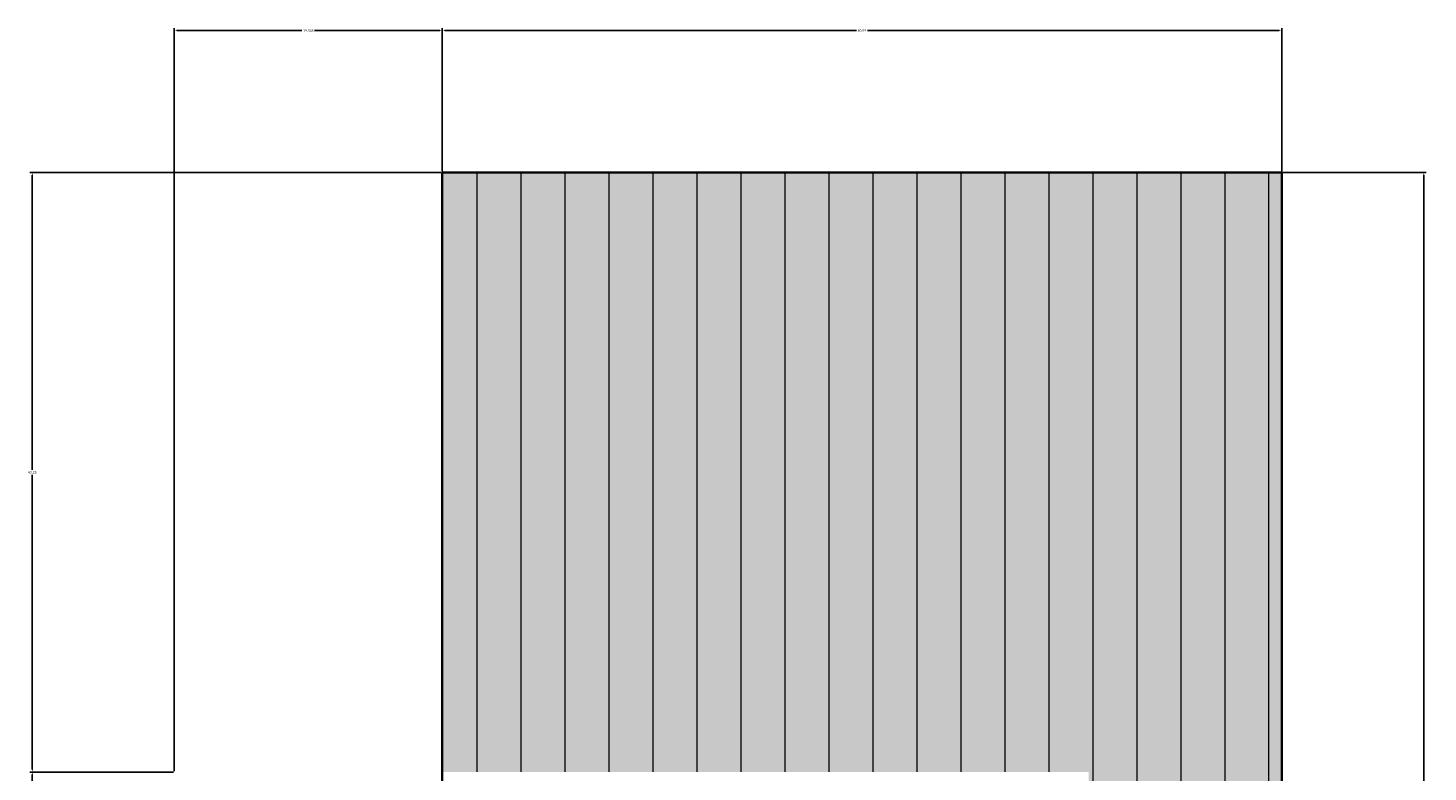
# Model space of a CAD drawing. Units: millimetres. Extents: x 446512 to 447461, y 70395 to 70610.
# Tile 27 of 39: x 446954 to 447055, y 70556 to 70610. Entities that reach past the tile are written whole.
import ezdxf

# ---------------------------------------------------------------- set-up
doc = ezdxf.new("R2010")
doc.units = ezdxf.units.MM
for name, color, linetype, lineweight in [('A-ANNO-DIMS', 2, 'Continuous', 18), ('A-FURN', 7, 'Continuous', 35), ('A-FURN-PATT', 38, 'Continuous', 13)]:
    doc.layers.add(name, color=color, linetype=linetype, lineweight=lineweight)
doc.styles.get("Standard").update_dxf_attribs({"font": 'arial.ttf'})
doc.dimstyles.get("Standard").update_dxf_attribs({"dimtxt": 0.18, "dimasz": 0.18, "dimexe": 0.18, "dimexo": 0.0625, "dimgap": 0.09, "dimtad": 0, "dimtih": 1, "dimtoh": 1, "dimdec": 4, "dimzin": 0, "dimdsep": 46, "dimtxsty": 'Standard', "dimcen": 0.09, "dimadec": 0, "dimazin": 0, "dimtfac": 1, "dimtdec": 4, "dimtofl": 0, "dimtmove": 0, "dimatfit": 3, "dimfxl": 1, "dimtolj": 1, "dimtzin": 0, "dimarcsym": 0})

# ---------------------------------------------------------------- blocks, each defined once
blk = doc.blocks.new('*D50')
at = {"layer": 'A-ANNO-DIMS', "color": 0, "lineweight": -2, "transparency": 16777216}
for p, q in [((446964.17, 70556.51), (446964.17, 70610.14)), ((446964.35, 70609.96), (446973.38, 70609.96)), ((446983.33, 70609.96), (446974.29, 70609.96)), ((446983.51, 70599.78), (446983.51, 70610.14))]:
    blk.add_line(p, q, dxfattribs=at)
at = {"layer": 'A-ANNO-DIMS', "color": 0, "transparency": 16777216}
for points in [[(446964.35, 70609.99), (446964.35, 70609.93), (446964.17, 70609.96)], [(446983.33, 70609.99), (446983.33, 70609.93), (446983.51, 70609.96)]]:
    blk.add_solid(points, dxfattribs=at)
at = {"layer": 'Defpoints', "color": 0, "transparency": 16777216}
for p in [(446983.51, 70609.96), (446983.51, 70599.71), (446964.17, 70556.45)]:
    blk.add_point(p, dxfattribs=at)
at = {"layer": 'A-ANNO-DIMS', "color": 0, "transparency": 16777216, "insert": (446973.84, 70609.96), "char_height": 0.18, "attachment_point": 5}
blk.add_mtext('\\A1;19.338', dxfattribs=at)
blk = doc.blocks.new('*D51')
at = {"layer": 'A-ANNO-DIMS', "color": 0, "lineweight": -2, "transparency": 16777216}
for p, q in [((446983.51, 70599.78), (446983.51, 70610.14)), ((446983.69, 70609.96), (447013.41, 70609.96)), ((447043.92, 70609.96), (447014.2, 70609.96)), ((447044.1, 70599.78), (447044.1, 70610.14))]:
    blk.add_line(p, q, dxfattribs=at)
at = {"layer": 'A-ANNO-DIMS', "color": 0, "transparency": 16777216}
for points in [[(446983.69, 70609.99), (446983.69, 70609.93), (446983.51, 70609.96)], [(447043.92, 70609.99), (447043.92, 70609.93), (447044.1, 70609.96)]]:
    blk.add_solid(points, dxfattribs=at)
at = {"layer": 'Defpoints', "color": 0, "transparency": 16777216}
for p in [(447044.1, 70609.96), (446983.51, 70599.71), (447044.1, 70599.71)]:
    blk.add_point(p, dxfattribs=at)
at = {"layer": 'A-ANNO-DIMS', "color": 0, "transparency": 16777216, "insert": (447013.8, 70609.96), "char_height": 0.18, "attachment_point": 5}
blk.add_mtext('\\A1;60.59', dxfattribs=at)
blk = doc.blocks.new('*D52')
at = {"layer": 'A-ANNO-DIMS', "color": 0, "lineweight": -2, "transparency": 16777216}
for p, q in [((447044.16, 70599.71), (447054.53, 70599.71)), ((447054.35, 70599.53), (447054.35, 70502.7)), ((447054.35, 70405.49), (447054.35, 70502.33)), ((447044.16, 70405.31), (447054.53, 70405.31))]:
    blk.add_line(p, q, dxfattribs=at)
at = {"layer": 'A-ANNO-DIMS', "color": 0, "transparency": 16777216}
for points in [[(447054.32, 70599.53), (447054.38, 70599.53), (447054.35, 70599.71)], [(447054.32, 70405.49), (447054.38, 70405.49), (447054.35, 70405.31)]]:
    blk.add_solid(points, dxfattribs=at)
at = {"layer": 'Defpoints', "color": 0, "transparency": 16777216}
for p in [(447044.1, 70599.71), (447054.35, 70599.71), (447044.1, 70405.31)]:
    blk.add_point(p, dxfattribs=at)
at = {"layer": 'A-ANNO-DIMS', "color": 0, "transparency": 16777216, "insert": (447054.35, 70502.51), "char_height": 0.18, "attachment_point": 5}
blk.add_mtext('\\A1;194.4', dxfattribs=at)
blk = doc.blocks.new('*D54')
at = {"layer": 'A-ANNO-DIMS', "color": 0, "lineweight": -2, "transparency": 16777216}
for p, q in [((446964.11, 70556.45), (446953.74, 70556.45)), ((446953.92, 70556.27), (446953.92, 70499.63)), ((446953.92, 70442.63), (446953.92, 70499.27)), ((446964.11, 70442.45), (446953.74, 70442.45))]:
    blk.add_line(p, q, dxfattribs=at)
at = {"layer": 'A-ANNO-DIMS', "color": 0, "transparency": 16777216}
for points in [[(446953.89, 70556.27), (446953.95, 70556.27), (446953.92, 70556.45)], [(446953.89, 70442.63), (446953.95, 70442.63), (446953.92, 70442.45)]]:
    blk.add_solid(points, dxfattribs=at)
at = {"layer": 'Defpoints', "color": 0, "transparency": 16777216}
for p in [(446953.92, 70556.45), (446964.17, 70556.45), (446964.17, 70442.45)]:
    blk.add_point(p, dxfattribs=at)
at = {"layer": 'A-ANNO-DIMS', "color": 0, "transparency": 16777216, "insert": (446953.92, 70499.45), "char_height": 0.18, "attachment_point": 5}
blk.add_mtext('\\A1;114', dxfattribs=at)
blk = doc.blocks.new('*D55')
at = {"layer": 'A-ANNO-DIMS', "color": 0, "lineweight": -2, "transparency": 16777216}
for p, q in [((446983.44, 70599.71), (446953.74, 70599.71)), ((446953.92, 70599.53), (446953.92, 70578.26)), ((446953.92, 70556.63), (446953.92, 70577.9)), ((446964.11, 70556.45), (446953.74, 70556.45))]:
    blk.add_line(p, q, dxfattribs=at)
at = {"layer": 'A-ANNO-DIMS', "color": 0, "transparency": 16777216}
for points in [[(446953.89, 70599.53), (446953.95, 70599.53), (446953.92, 70599.71)], [(446953.89, 70556.63), (446953.95, 70556.63), (446953.92, 70556.45)]]:
    blk.add_solid(points, dxfattribs=at)
at = {"layer": 'Defpoints', "color": 0, "transparency": 16777216}
for p in [(446953.92, 70599.71), (446983.51, 70599.71), (446964.17, 70556.45)]:
    blk.add_point(p, dxfattribs=at)
at = {"layer": 'A-ANNO-DIMS', "color": 0, "transparency": 16777216, "insert": (446953.92, 70578.08), "char_height": 0.18, "attachment_point": 5}
blk.add_mtext('\\A1;43.26', dxfattribs=at)
blk = doc.blocks.new('*D60')
at = {"layer": 'A-ANNO-DIMS', "color": 0, "lineweight": -2, "transparency": 16777216}
for p, q in [((446964.11, 70556.45), (446953.74, 70556.45)), ((446953.92, 70556.27), (446953.92, 70552.13)), ((446953.92, 70547.63), (446953.92, 70551.77)), ((446973.11, 70547.45), (446953.74, 70547.45))]:
    blk.add_line(p, q, dxfattribs=at)
at = {"layer": 'A-ANNO-DIMS', "color": 0, "transparency": 16777216}
for points in [[(446953.89, 70556.27), (446953.95, 70556.27), (446953.92, 70556.45)], [(446953.89, 70547.63), (446953.95, 70547.63), (446953.92, 70547.45)]]:
    blk.add_solid(points, dxfattribs=at)
at = {"layer": 'Defpoints', "color": 0, "transparency": 16777216}
for p in [(446953.92, 70556.45), (446964.17, 70556.45), (446973.17, 70547.45)]:
    blk.add_point(p, dxfattribs=at)
at = {"layer": 'A-ANNO-DIMS', "color": 0, "transparency": 16777216, "insert": (446953.92, 70551.95), "char_height": 0.18, "attachment_point": 5}
blk.add_mtext('\\A1;9', dxfattribs=at)

msp = doc.modelspace()

# ---------------------------------------------------------------- hatches: boundary and pattern name
at = {"layer": 'A-FURN-PATT'}
h = msp.add_hatch(dxfattribs=at)
h.set_pattern_fill('ANSI31', color=256, angle=45)
h.paths.add_polyline_path([(447044.0961, 70599.7147), (446983.5069, 70599.7147), (446983.5069, 70556.4508), (447030.1693, 70556.4508), (447030.1693, 70442.4508), (446983.5069, 70442.4508), (446983.5069, 70405.3145), (447044.0961, 70405.3145)])
h.paths.add_polyline_path([(447021.1693, 70547.4508), (446983.5069, 70547.4508), (446983.5069, 70451.4508), (447021.1693, 70451.4508)], flags=17)
h = msp.add_hatch(color=256, dxfattribs=at)
h.dxf.hatch_style = 1
h.paths.add_polyline_path([(447021.1693, 70483.6935), (446983.5069, 70483.6935), (446983.5069, 70479.6272), (447021.1693, 70479.6272)], flags=17)
h.paths.add_polyline_path([(447030.1693, 70483.6935), (447021.1693, 70483.6935), (447021.1693, 70479.6272), (447030.1693, 70479.6272)], flags=17)
h.paths.add_polyline_path([(447044.0961, 70599.7147), (446983.5069, 70599.7147), (446983.5069, 70556.4508), (447030.1693, 70556.4508), (447030.1693, 70442.4508), (446983.5069, 70442.4508), (446983.5069, 70405.3145), (447044.0961, 70405.3145)])

# ---------------------------------------------------------------- linework, layer by layer
at = {"layer": 'A-FURN'}
for p, q in [((447044.0961, 70599.7147), (446983.5069, 70599.7147)), ((446983.5069, 70599.7147), (446983.5069, 70405.3145)), ((447044.0961, 70405.3145), (447044.0961, 70599.7147))]:
    msp.add_line(p, q, dxfattribs=at)

# ---------------------------------------------------------------- dimensions: what is measured, and where the dimension line sits
at = {"layer": 'A-ANNO-DIMS'}
for base, p1, p2, override, picture, middle in [((446983.5069, 70609.9647), (446964.1693, 70556.4508), (446983.5069, 70599.7147), {"dimdec": 3, "dimlfac": 1, "dimrnd": 0, "dimzin": 0, "dimdsep": 46, "dimlunit": 2}, '*D50', (446973.8381, 70609.9647)), ((447044.0961, 70609.9647), (446983.5069, 70599.7147), (447044.0961, 70599.7147), {"dimdec": 2, "dimlfac": 1, "dimrnd": 0, "dimzin": 0, "dimdsep": 46, "dimlunit": 2}, '*D51', (447013.8015, 70609.9647))]:
    dim = msp.add_linear_dim(base=base, p1=p1, p2=p2, dimstyle='Standard', override=override, dxfattribs=at)
    dim.commit()
    dim.dimension.update_dxf_attribs({"geometry": picture, "text_midpoint": middle})
for base, p1, p2, override, picture, middle in [((446953.9193, 70599.7147), (446964.1693, 70556.4508), (446983.5069, 70599.7147), {"dimdec": 2, "dimlfac": 1, "dimrnd": 0, "dimzin": 0, "dimdsep": 46, "dimlunit": 2}, '*D55', (446953.9193, 70578.0827)), ((447054.3461, 70599.7147), (447044.0961, 70405.3145), (447044.0961, 70599.7147), {"dimdec": 1, "dimlfac": 1, "dimrnd": 0, "dimzin": 0, "dimdsep": 46, "dimlunit": 2}, '*D52', (447054.3461, 70502.5146)), ((446953.9193, 70556.4508), (446964.1693, 70442.4508), (446964.1693, 70556.4508), {"dimdec": 0, "dimlfac": 1, "dimrnd": 0, "dimzin": 0, "dimdsep": 46, "dimlunit": 2}, '*D54', (446953.9193, 70499.4508)), ((446953.9193, 70556.4508), (446973.1693, 70547.4508), (446964.1693, 70556.4508), {"dimdec": 0, "dimlfac": 1, "dimrnd": 0, "dimzin": 0, "dimdsep": 46, "dimlunit": 2}, '*D60', (446953.9193, 70551.9508))]:
    dim = msp.add_linear_dim(base=base, p1=p1, p2=p2, angle=90, dimstyle='Standard', override=override, dxfattribs=at)
    dim.commit()
    dim.dimension.update_dxf_attribs({"geometry": picture, "text_midpoint": middle})

doc.saveas('drawing.dxf')
